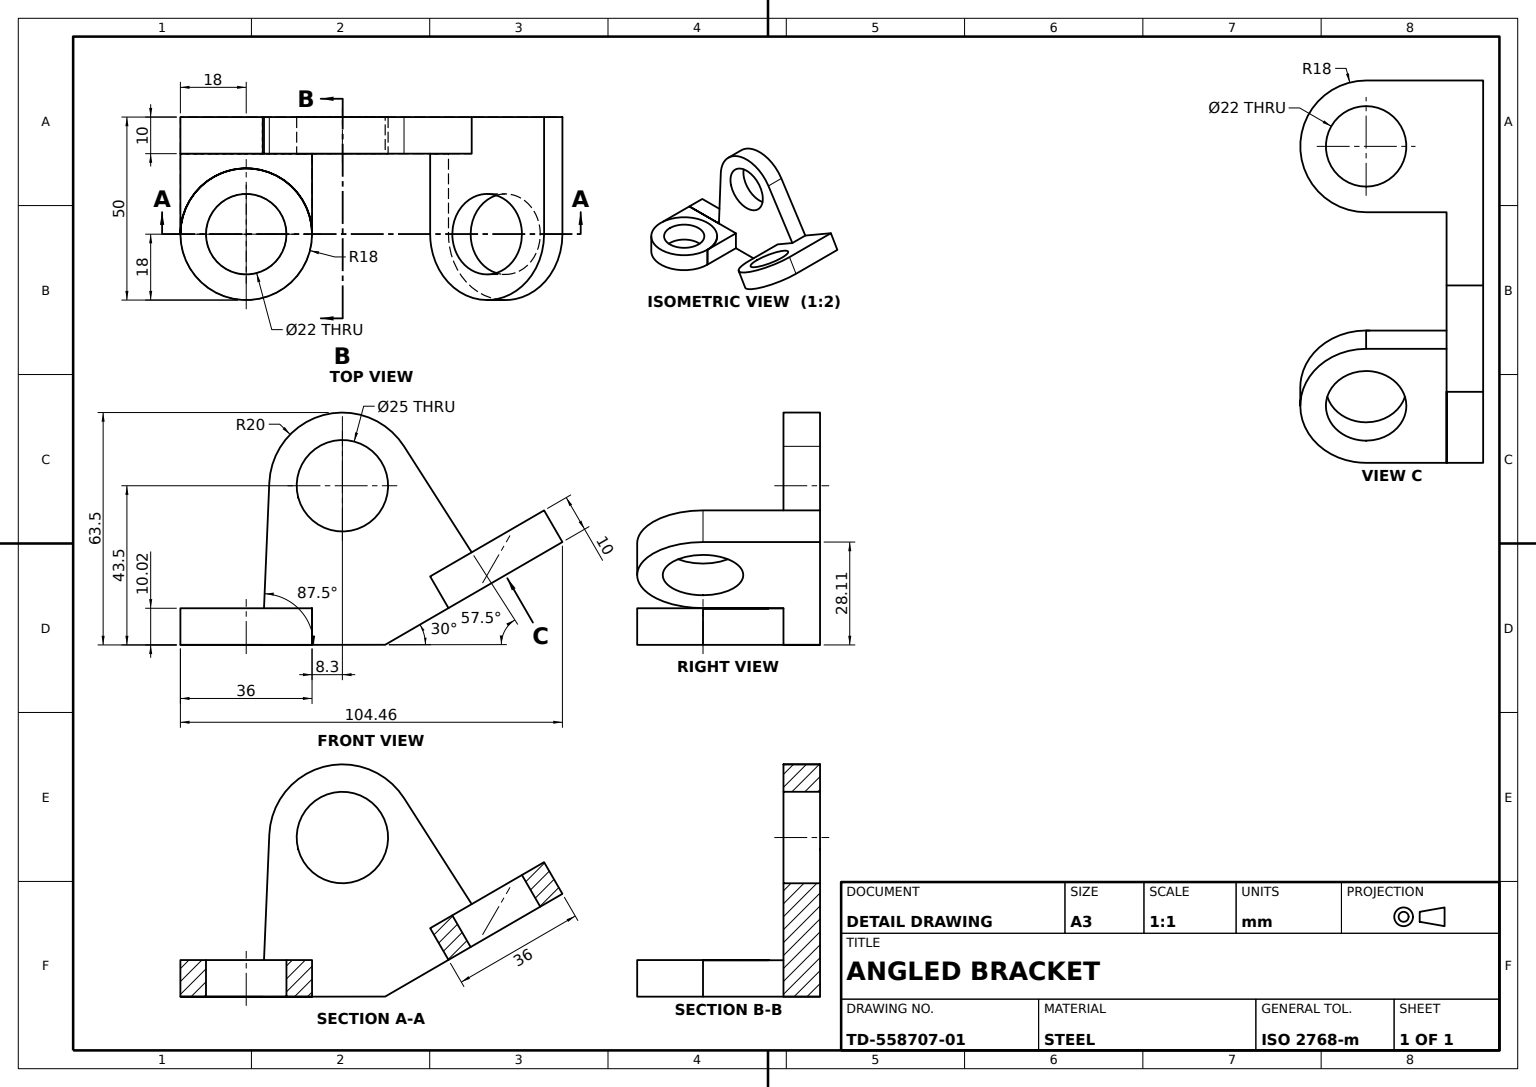
from build123d import *

# Parameters (mm, degrees)
LUG_PLATE_DEPTH          = 10
FLANGE_BASE_DEPTH        = 10
ANGLED_FLANGE_ARMS_DEPTH = 22
EYE_BOSS_A_SKETCH_R      = 18.000000011
EYE_BOSS_A_DEPTH         = 10
EYE_BOSS_B_SKETCH_R      = 18
EYE_BOSS_B_DEPTH         = 10
EYE_HOLE_A_22_SKETCH_R   = 11
EYE_HOLE_A_22_DEPTH      = 10
EYE_HOLE_B_22_SKETCH_R   = 11
EYE_HOLE_B_22_DEPTH      = 10
LUG_BORE_25_SKETCH_R     = 12.5
LUG_BORE_25_DEPTH        = 10


with BuildPart() as part:
    # Lug Plate Sketch → Lug Plate (new body)
    with BuildSketch(Plane.XY):
        with BuildLine():
            Line((-19.074339015, 51.01411599), (-32.420050634, 8.686926386))
            Line((-32.420050634, 8.686926386), (0, 0))
            Line((0, 0), (32.420050634, 8.686926386))
            Line((32.420050634, 8.686926386), (19.074339015, 51.01411599))
            ThreePointArc((19.074339015, 51.01411599), (0, 65), (-19.074339015, 51.01411599))
        make_face()
    extrude(amount=LUG_PLATE_DEPTH)

    # Flange Base Sketch → Flange Base (add)
    with BuildSketch(Plane.XY.offset(10)):
        Polygon((-54.079171789, 14.541040303), (-32.414511502, 8.704494269), (-29.410127859, 18.233181813), (-51.490581609, 24.149621564), align=None)
        Polygon((-32.414511502, 8.704494269), (-19.318516526, 5.176380902), (-16.730326075, 14.835639165), (-29.410127859, 18.233181813), align=None)
        Polygon((16.730326075, 14.835639165), (19.318516526, 5.176380902), (32.420050634, 8.686926386), (29.410127859, 18.233181813), align=None)
        Polygon((29.410127859, 18.233181813), (32.420050634, 8.686926386), (54.091846272, 14.493866526), (51.503655821, 24.153124789), align=None)
    extrude(amount=-FLANGE_BASE_DEPTH)

    # Angled Flange Arms Sketch → Angled Flange Arms (add)
    with BuildSketch(Plane.XY.offset(10)):
        Polygon((-51.490581609, 24.149621564), (-16.729926347, 14.784962163), (-19.318186451, 5.177606105), (-54.079171789, 14.541040303), align=None)
        Polygon((51.503655821, 24.153124789), (16.730326075, 14.835639165), (19.318516526, 5.176380902), (54.091846272, 14.493866526), align=None)
    extrude(amount=ANGLED_FLANGE_ARMS_DEPTH)

    # Eye Boss A Sketch → Eye Boss A (add)
    with BuildSketch(Plane(origin=(-0.006544851, -0.024297225, 0), x_dir=(0.965582925438563, -0.2600953942335516, 0), z_dir=(-0.2600953942335516, -0.9655829254385631, 0))):
        with Locations((-37.9999825, 32)):
            Circle(EYE_BOSS_A_SKETCH_R)
    extrude(amount=-EYE_BOSS_A_DEPTH)

    # Eye Boss B Sketch → Eye Boss B (add)
    with BuildSketch(Plane(origin=(0, 0, 0), x_dir=(0.9659258262890681, 0.25881904510252146, 0), z_dir=(0.25881904510252146, -0.9659258262890681, 0))):
        with Locations((38, 32)):
            Circle(EYE_BOSS_B_SKETCH_R)
    extrude(amount=-EYE_BOSS_B_DEPTH)

    # Eye Hole A _22 Sketch → Eye Hole A _22 (cut)
    with BuildSketch(Plane(origin=(-0.006544851, -0.024297225, 0), x_dir=(0.965582925438563, -0.2600953942335516, 0), z_dir=(-0.2600953942335516, -0.9655829254385631, 0))):
        with Locations((-37.9999825, 32)):
            Circle(EYE_HOLE_A_22_SKETCH_R)
    extrude(amount=-EYE_HOLE_A_22_DEPTH, mode=Mode.SUBTRACT)

    # Eye Hole B _22 Sketch → Eye Hole B _22 (cut)
    with BuildSketch(Plane(origin=(0, 0, 0), x_dir=(0.9659258262890681, 0.25881904510252146, 0), z_dir=(0.25881904510252146, -0.9659258262890681, 0))):
        with Locations((38, 32)):
            Circle(EYE_HOLE_B_22_SKETCH_R)
    extrude(amount=-EYE_HOLE_B_22_DEPTH, mode=Mode.SUBTRACT)

    # Lug Bore _25 Sketch → Lug Bore _25 (cut)
    with BuildSketch(Plane.XY.offset(10)):
        with Locations((0, 45)):
            Circle(LUG_BORE_25_SKETCH_R)
    extrude(amount=-LUG_BORE_25_DEPTH, mode=Mode.SUBTRACT)


solid = part.part
